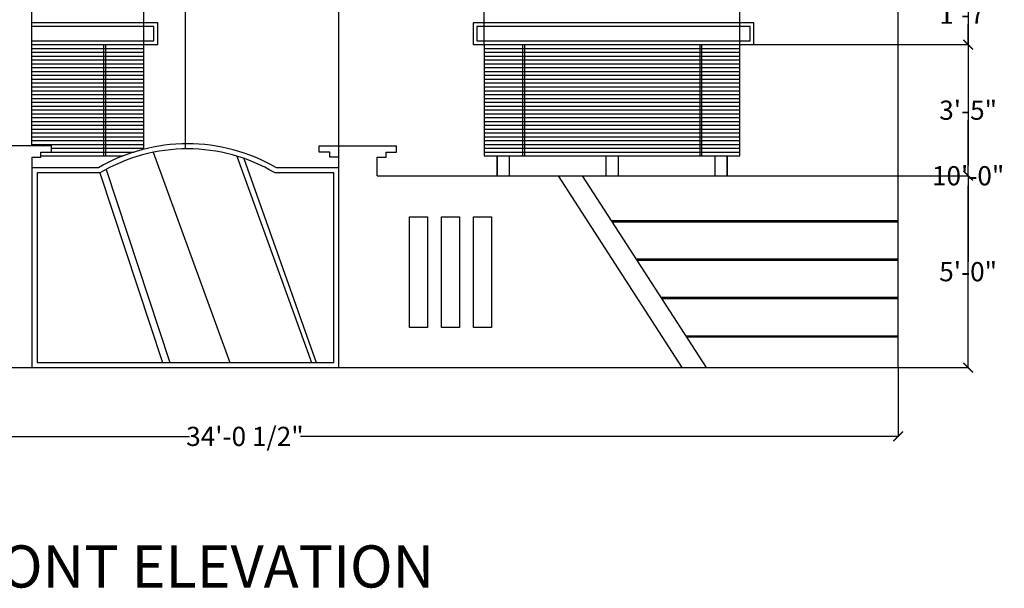
# Model space of a CAD drawing. Units: inches. Extents: x 2278 to 7495, y -71 to 1198.
# Tile 9 of 44: x 4871 to 5179, y -71 to 107. Entities that reach past the tile are written whole.
import ezdxf

# ---------------------------------------------------------------- set-up
doc = ezdxf.new("R2010")
doc.units = ezdxf.units.IN
doc.header["$MEASUREMENT"] = 0
for name, color, linetype, lineweight in [('A-ANNO-DIMS', 2, 'Continuous', 18), ('A-ANNO-TEXT', 7, 'Continuous', 25), ('A-ELEV', 7, 'Continuous', 25)]:
    doc.layers.add(name, color=color, linetype=linetype, lineweight=lineweight)
doc.styles.get("Standard").update_dxf_attribs({"font": 'arial.ttf'})
doc.dimstyles.get("Standard").update_dxf_attribs({"dimtxt": 6, "dimasz": 3, "dimexe": 0.18, "dimexo": 0.0625, "dimgap": 0.09, "dimtad": 0, "dimtih": 1, "dimtoh": 1, "dimdec": 0, "dimzin": 0, "dimdsep": 46, "dimlunit": 3, "dimtxsty": 'Standard', "dimblk": 'ARCHTICK', "dimcen": 0.09, "dimadec": 0, "dimazin": 0, "dimtfac": 1, "dimtdec": 0, "dimtofl": 0, "dimtmove": 0, "dimatfit": 3, "dimfxl": 1, "dimtolj": 1, "dimtzin": 0, "dimarcsym": 0})

# ---------------------------------------------------------------- blocks, each defined once
blk = doc.blocks.new('_ArchTick')
at = {"color": 0, "linetype": 'ByBlock', "const_width": 0.15}
blk.add_lwpolyline([(-0.5, -0.5), (0.5, 0.5)], dxfattribs=at)
blk = doc.blocks.new('*D123')
at = {"layer": 'A-ANNO-DIMS', "color": 0, "lineweight": -2, "transparency": 16777216}
for p, q in [((4736.95, 340.16), (4736.95, -23.43)), ((5145.68, -1.81), (5145.68, -23.43)), ((4736.95, -23.25), (4923.93, -23.25)), ((5145.68, -23.25), (4958.7, -23.25))]:
    blk.add_line(p, q, dxfattribs=at)
at = {"layer": 'Defpoints', "color": 0, "transparency": 16777216}
for p in [(4736.95, 340.22), (5145.68, -1.75), (5145.68, -23.25)]:
    blk.add_point(p, dxfattribs=at)
at = {"layer": 'A-ANNO-DIMS', "color": 0, "lineweight": -2, "transparency": 16777216, "xscale": 3, "yscale": 3, "zscale": 3, "rotation": 180}
blk.add_blockref('_ArchTick', (4736.95, -23.25), dxfattribs=at)
at = {"layer": 'A-ANNO-DIMS', "color": 0, "lineweight": -2, "transparency": 16777216, "xscale": 3, "yscale": 3, "zscale": 3}
blk.add_blockref('_ArchTick', (5145.68, -23.25), dxfattribs=at)
at = {"layer": 'A-ANNO-DIMS', "color": 0, "transparency": 16777216, "insert": (4941.31, -23.25), "char_height": 6, "attachment_point": 5}
blk.add_mtext('\\A1;34\'-0 1/2"', dxfattribs=at)
blk = doc.blocks.new('*D126')
at = {"layer": 'A-ANNO-DIMS', "color": 0, "lineweight": -2, "transparency": 16777216}
for p, q in [((4837.74, 313.27), (4837.74, 361.9)), ((4837.74, 361.72), (4848.14, 361.72)), ((4874.68, 361.72), (4864.27, 361.72)), ((4874.68, 99.32), (4874.68, 361.9))]:
    blk.add_line(p, q, dxfattribs=at)
at = {"layer": 'Defpoints', "color": 0, "transparency": 16777216}
for p in [(4874.68, 361.72), (4837.74, 313.21), (4874.68, 99.25)]:
    blk.add_point(p, dxfattribs=at)
at = {"layer": 'A-ANNO-DIMS', "color": 0, "lineweight": -2, "transparency": 16777216, "xscale": 3, "yscale": 3, "zscale": 3, "rotation": 180}
blk.add_blockref('_ArchTick', (4837.74, 361.72), dxfattribs=at)
at = {"layer": 'A-ANNO-DIMS', "color": 0, "lineweight": -2, "transparency": 16777216, "xscale": 3, "yscale": 3, "zscale": 3}
blk.add_blockref('_ArchTick', (4874.68, 361.72), dxfattribs=at)
at = {"layer": 'A-ANNO-DIMS', "color": 0, "transparency": 16777216, "insert": (4856.21, 361.72), "char_height": 6, "attachment_point": 5}
blk.add_mtext('\\A1;3\'-1"', dxfattribs=at)
blk = doc.blocks.new('*D127')
at = {"layer": 'A-ANNO-DIMS', "color": 0, "lineweight": -2, "transparency": 16777216}
for p, q in [((4874.68, 99.32), (4874.68, 361.9)), ((4874.68, 361.72), (4881.73, 361.72)), ((4909.68, 361.72), (4902.62, 361.72)), ((4909.68, 99.32), (4909.68, 361.9))]:
    blk.add_line(p, q, dxfattribs=at)
at = {"layer": 'Defpoints', "color": 0, "transparency": 16777216}
for p in [(4909.68, 361.72), (4874.68, 99.25), (4909.68, 99.25)]:
    blk.add_point(p, dxfattribs=at)
at = {"layer": 'A-ANNO-DIMS', "color": 0, "lineweight": -2, "transparency": 16777216, "xscale": 3, "yscale": 3, "zscale": 3, "rotation": 180}
blk.add_blockref('_ArchTick', (4874.68, 361.72), dxfattribs=at)
at = {"layer": 'A-ANNO-DIMS', "color": 0, "lineweight": -2, "transparency": 16777216, "xscale": 3, "yscale": 3, "zscale": 3}
blk.add_blockref('_ArchTick', (4909.68, 361.72), dxfattribs=at)
at = {"layer": 'A-ANNO-DIMS', "color": 0, "transparency": 16777216, "insert": (4892.18, 361.72), "char_height": 6, "attachment_point": 5}
blk.add_mtext('\\A1;2\'-11"', dxfattribs=at)
blk = doc.blocks.new('*D128')
at = {"layer": 'A-ANNO-DIMS', "color": 0, "lineweight": -2, "transparency": 16777216}
for p, q in [((4909.68, 99.32), (4909.68, 361.9)), ((4909.68, 361.72), (4932.11, 361.72)), ((4970.68, 361.72), (4948.24, 361.72)), ((4970.68, 60.78), (4970.68, 361.9))]:
    blk.add_line(p, q, dxfattribs=at)
at = {"layer": 'Defpoints', "color": 0, "transparency": 16777216}
for p in [(4970.68, 361.72), (4909.68, 99.25), (4970.68, 60.72)]:
    blk.add_point(p, dxfattribs=at)
at = {"layer": 'A-ANNO-DIMS', "color": 0, "lineweight": -2, "transparency": 16777216, "xscale": 3, "yscale": 3, "zscale": 3, "rotation": 180}
blk.add_blockref('_ArchTick', (4909.68, 361.72), dxfattribs=at)
at = {"layer": 'A-ANNO-DIMS', "color": 0, "lineweight": -2, "transparency": 16777216, "xscale": 3, "yscale": 3, "zscale": 3}
blk.add_blockref('_ArchTick', (4970.68, 361.72), dxfattribs=at)
at = {"layer": 'A-ANNO-DIMS', "color": 0, "transparency": 16777216, "insert": (4940.18, 361.72), "char_height": 6, "attachment_point": 5}
blk.add_mtext('\\A1;5\'-1"', dxfattribs=at)
blk = doc.blocks.new('*D129')
at = {"layer": 'A-ANNO-DIMS', "color": 0, "lineweight": -2, "transparency": 16777216}
for p, q in [((4970.68, 60.78), (4970.68, 361.9)), ((4970.68, 361.72), (4978.37, 361.72)), ((5016.18, 361.72), (5008.48, 361.72)), ((5016.18, 99.32), (5016.18, 361.9))]:
    blk.add_line(p, q, dxfattribs=at)
at = {"layer": 'Defpoints', "color": 0, "transparency": 16777216}
for p in [(5016.18, 361.72), (5016.18, 99.25), (4970.68, 60.72)]:
    blk.add_point(p, dxfattribs=at)
at = {"layer": 'A-ANNO-DIMS', "color": 0, "lineweight": -2, "transparency": 16777216, "xscale": 3, "yscale": 3, "zscale": 3, "rotation": 180}
blk.add_blockref('_ArchTick', (4970.68, 361.72), dxfattribs=at)
at = {"layer": 'A-ANNO-DIMS', "color": 0, "lineweight": -2, "transparency": 16777216, "xscale": 3, "yscale": 3, "zscale": 3}
blk.add_blockref('_ArchTick', (5016.18, 361.72), dxfattribs=at)
at = {"layer": 'A-ANNO-DIMS', "color": 0, "transparency": 16777216, "insert": (4993.43, 361.72), "char_height": 6, "attachment_point": 5}
blk.add_mtext('\\A1;3\'-9 1/2"', dxfattribs=at)
blk = doc.blocks.new('*D130')
at = {"layer": 'A-ANNO-DIMS', "color": 0, "lineweight": -2, "transparency": 16777216}
for p, q in [((5016.18, 99.32), (5016.18, 361.9)), ((5016.18, 361.72), (5048.1, 361.72)), ((5096.18, 361.72), (5064.26, 361.72)), ((5096.18, 99.32), (5096.18, 361.9))]:
    blk.add_line(p, q, dxfattribs=at)
at = {"layer": 'Defpoints', "color": 0, "transparency": 16777216}
for p in [(5096.18, 361.72), (5016.18, 99.25), (5096.18, 99.25)]:
    blk.add_point(p, dxfattribs=at)
at = {"layer": 'A-ANNO-DIMS', "color": 0, "lineweight": -2, "transparency": 16777216, "xscale": 3, "yscale": 3, "zscale": 3, "rotation": 180}
blk.add_blockref('_ArchTick', (5016.18, 361.72), dxfattribs=at)
at = {"layer": 'A-ANNO-DIMS', "color": 0, "lineweight": -2, "transparency": 16777216, "xscale": 3, "yscale": 3, "zscale": 3}
blk.add_blockref('_ArchTick', (5096.18, 361.72), dxfattribs=at)
at = {"layer": 'A-ANNO-DIMS', "color": 0, "transparency": 16777216, "insert": (5056.18, 361.72), "char_height": 6, "attachment_point": 5}
blk.add_mtext('\\A1;6\'-8"', dxfattribs=at)
blk = doc.blocks.new('*D131')
at = {"layer": 'A-ANNO-DIMS', "color": 0, "lineweight": -2, "transparency": 16777216}
for p, q in [((5096.18, 99.32), (5096.18, 361.9)), ((5096.18, 361.72), (5105.75, 361.72)), ((5145.68, 361.72), (5136.1, 361.72)), ((5145.68, 118.32), (5145.68, 361.9))]:
    blk.add_line(p, q, dxfattribs=at)
at = {"layer": 'Defpoints', "color": 0, "transparency": 16777216}
for p in [(5145.68, 361.72), (5145.68, 118.25), (5096.18, 99.25)]:
    blk.add_point(p, dxfattribs=at)
at = {"layer": 'A-ANNO-DIMS', "color": 0, "lineweight": -2, "transparency": 16777216, "xscale": 3, "yscale": 3, "zscale": 3, "rotation": 180}
blk.add_blockref('_ArchTick', (5096.18, 361.72), dxfattribs=at)
at = {"layer": 'A-ANNO-DIMS', "color": 0, "lineweight": -2, "transparency": 16777216, "xscale": 3, "yscale": 3, "zscale": 3}
blk.add_blockref('_ArchTick', (5145.68, 361.72), dxfattribs=at)
at = {"layer": 'A-ANNO-DIMS', "color": 0, "transparency": 16777216, "insert": (5120.93, 361.72), "char_height": 6, "attachment_point": 5}
blk.add_mtext('\\A1;4\'-1 1/2"', dxfattribs=at)
blk = doc.blocks.new('*D136')
at = {"layer": 'A-ANNO-DIMS', "color": 0, "lineweight": -2, "transparency": 16777216}
for p, q in [((5145.74, 58.25), (5167.75, 58.25)), ((5167.57, 58.25), (5167.57, 31.41)), ((5167.57, -1.75), (5167.57, 25.1)), ((5145.74, -1.75), (5167.75, -1.75))]:
    blk.add_line(p, q, dxfattribs=at)
at = {"layer": 'Defpoints', "color": 0, "transparency": 16777216}
for p in [(5145.68, 58.25), (5167.57, 58.25), (5145.68, -1.75)]:
    blk.add_point(p, dxfattribs=at)
at = {"layer": 'A-ANNO-DIMS', "color": 0, "lineweight": -2, "transparency": 16777216, "xscale": 3, "yscale": 3, "zscale": 3}
for p, rotation in [((5167.57, 58.25), 90), ((5167.57, -1.75), 270)]:
    blk.add_blockref('_ArchTick', p, dxfattribs=dict(at, rotation=rotation))
at = {"layer": 'A-ANNO-DIMS', "color": 0, "transparency": 16777216, "insert": (5167.57, 28.25), "char_height": 6, "attachment_point": 5}
blk.add_mtext('\\A1;5\'-0"', dxfattribs=at)
blk = doc.blocks.new('*D137')
at = {"layer": 'A-ANNO-DIMS', "color": 0, "lineweight": -2, "transparency": 16777216}
for p, q in [((5096.24, 99.25), (5167.75, 99.25)), ((5167.57, 99.25), (5167.57, 81.91)), ((5167.57, 58.25), (5167.57, 75.6)), ((5145.74, 58.25), (5167.75, 58.25))]:
    blk.add_line(p, q, dxfattribs=at)
at = {"layer": 'Defpoints', "color": 0, "transparency": 16777216}
for p in [(5096.18, 99.25), (5167.57, 99.25), (5145.68, 58.25)]:
    blk.add_point(p, dxfattribs=at)
at = {"layer": 'A-ANNO-DIMS', "color": 0, "lineweight": -2, "transparency": 16777216, "xscale": 3, "yscale": 3, "zscale": 3}
for p, rotation in [((5167.57, 99.25), 90), ((5167.57, 58.25), 270)]:
    blk.add_blockref('_ArchTick', p, dxfattribs=dict(at, rotation=rotation))
at = {"layer": 'A-ANNO-DIMS', "color": 0, "transparency": 16777216, "insert": (5167.57, 78.75), "char_height": 6, "attachment_point": 5}
blk.add_mtext('\\A1;3\'-5"', dxfattribs=at)
blk = doc.blocks.new('*D138')
at = {"layer": 'A-ANNO-DIMS', "color": 0, "lineweight": -2, "transparency": 16777216}
for p, q in [((5145.74, 118.25), (5167.75, 118.25)), ((5167.57, 118.25), (5167.57, 111.86)), ((5167.57, 99.25), (5167.57, 105.65)), ((5096.24, 99.25), (5167.75, 99.25))]:
    blk.add_line(p, q, dxfattribs=at)
at = {"layer": 'Defpoints', "color": 0, "transparency": 16777216}
for p in [(5145.68, 118.25), (5167.57, 118.25), (5096.18, 99.25)]:
    blk.add_point(p, dxfattribs=at)
at = {"layer": 'A-ANNO-DIMS', "color": 0, "lineweight": -2, "transparency": 16777216, "xscale": 3, "yscale": 3, "zscale": 3}
for p, rotation in [((5167.57, 118.25), 90), ((5167.57, 99.25), 270)]:
    blk.add_blockref('_ArchTick', p, dxfattribs=dict(at, rotation=rotation))
at = {"layer": 'A-ANNO-DIMS', "color": 0, "transparency": 16777216, "insert": (5167.57, 108.75), "char_height": 6, "attachment_point": 5}
blk.add_mtext('\\A1;1\'-7"', dxfattribs=at)
blk = doc.blocks.new('*D143')
at = {"layer": 'A-ANNO-DIMS', "color": 0, "lineweight": -2, "transparency": 16777216}
for p, q in [((5145.74, 118.25), (5167.75, 118.25)), ((5167.57, 118.25), (5167.57, 61.41)), ((5167.57, -1.75), (5167.57, 55.1)), ((5145.74, -1.75), (5167.75, -1.75))]:
    blk.add_line(p, q, dxfattribs=at)
at = {"layer": 'Defpoints', "color": 0, "transparency": 16777216}
for p in [(5145.68, 118.25), (5167.57, 118.25), (5145.68, -1.75)]:
    blk.add_point(p, dxfattribs=at)
at = {"layer": 'A-ANNO-DIMS', "color": 0, "lineweight": -2, "transparency": 16777216, "xscale": 3, "yscale": 3, "zscale": 3}
for p, rotation in [((5167.57, 118.25), 90), ((5167.57, -1.75), 270)]:
    blk.add_blockref('_ArchTick', p, dxfattribs=dict(at, rotation=rotation))
at = {"layer": 'A-ANNO-DIMS', "color": 0, "transparency": 16777216, "insert": (5167.57, 58.25), "char_height": 6, "attachment_point": 5}
blk.add_mtext('\\A1;10\'-0"', dxfattribs=at)

msp = doc.modelspace()

# ---------------------------------------------------------------- linework, layer by layer
at = {"layer": 'A-ELEV'}
for p, q in [((4922.68, 66.66), (4922.68, 244.25)), ((5145.68, -1.75), (5145.68, 161.58)), ((4970.68, 67.61), (4970.68, 124.25)), ((4874.68, 67.61), (4874.68, 118.25)), ((4874.68, 99.25), (4909.68, 99.25)), ((4897.08, 99.25), (4897.08, 64.45)), ((4897.08, 99.25), (4897.08, 65.65)), ((4897.08, 99.25), (4897.08, 65.65)), ((4897.08, 99.25), (4897.08, 65.65)), ((4897.68, 99.25), (4897.68, 64.45)), ((4897.68, 99.25), (4897.68, 65.65)), ((4897.68, 99.25), (4897.68, 65.65)), ((4897.68, 99.25), (4897.68, 65.65)), ((4909.68, 66.54), (4909.68, 99.25)), ((5016.18, 99.25), (5096.18, 99.25)), ((5016.18, 99.25), (5016.18, 64.45)), ((5028.18, 99.25), (5028.18, 64.45)), ((5028.18, 99.25), (5028.18, 65.65)), ((5028.18, 99.25), (5028.18, 65.65)), ((5028.18, 99.25), (5028.18, 65.65)), ((5028.78, 99.25), (5028.78, 64.45)), ((5028.78, 99.25), (5028.78, 65.65)), ((5028.78, 99.25), (5028.78, 65.65)), ((5028.78, 99.25), (5028.78, 65.65)), ((5083.58, 99.25), (5083.58, 64.45)), ((5083.58, 99.25), (5083.58, 65.65)), ((5083.58, 99.25), (5083.58, 65.65)), ((5083.58, 99.25), (5083.58, 65.65)), ((5084.18, 99.25), (5084.18, 64.45)), ((5084.18, 99.25), (5084.18, 65.65)), ((5084.18, 99.25), (5084.18, 65.65)), ((5084.18, 99.25), (5084.18, 65.65)), ((5096.18, 64.45), (5096.18, 99.25)), ((4874.68, 98.05), (4909.68, 98.05)), ((4874.68, 96.85), (4909.68, 96.85)), ((4874.68, 95.65), (4909.68, 95.65)), ((5016.18, 98.05), (5096.18, 98.05)), ((5016.18, 96.85), (5096.18, 96.85)), ((5016.18, 95.65), (5096.18, 95.65)), ((4874.68, 94.45), (4909.68, 94.45)), ((4874.68, 93.25), (4909.68, 93.25)), ((5016.18, 94.45), (5096.18, 94.45)), ((5016.18, 93.25), (5096.18, 93.25)), ((4874.68, 92.05), (4909.68, 92.05)), ((4874.68, 90.85), (4909.68, 90.85)), ((4874.68, 89.65), (4909.68, 89.65)), ((5016.18, 92.05), (5096.18, 92.05)), ((5016.18, 90.85), (5096.18, 90.85)), ((5016.18, 89.65), (5096.18, 89.65)), ((4874.68, 88.45), (4909.68, 88.45)), ((4874.68, 87.25), (4909.68, 87.25)), ((5016.18, 88.45), (5096.18, 88.45)), ((5016.18, 87.25), (5096.18, 87.25)), ((4874.68, 86.05), (4909.68, 86.05)), ((4874.68, 84.85), (4909.68, 84.85)), ((4874.68, 83.65), (4909.68, 83.65)), ((5016.18, 86.05), (5096.18, 86.05)), ((5016.18, 84.85), (5096.18, 84.85)), ((5016.18, 83.65), (5096.18, 83.65)), ((4874.68, 82.45), (4909.68, 82.45)), ((4874.68, 81.25), (4909.68, 81.25)), ((5016.18, 82.45), (5096.18, 82.45)), ((5016.18, 81.25), (5096.18, 81.25)), ((4874.68, 80.05), (4909.68, 80.05)), ((4874.68, 78.85), (4909.68, 78.85)), ((4874.68, 77.65), (4909.68, 77.65)), ((5016.18, 80.05), (5096.18, 80.05)), ((5016.18, 78.85), (5096.18, 78.85)), ((5016.18, 77.65), (5096.18, 77.65)), ((4874.68, 76.45), (4909.68, 76.45)), ((4874.68, 75.25), (4909.68, 75.25)), ((4874.68, 74.05), (4909.68, 74.05)), ((5016.18, 76.45), (5096.18, 76.45)), ((5016.18, 75.25), (5096.18, 75.25)), ((5016.18, 74.05), (5096.18, 74.05)), ((4874.68, 72.85), (4909.68, 72.85)), ((4874.68, 71.65), (4909.68, 71.65)), ((5016.18, 72.85), (5096.18, 72.85)), ((5016.18, 71.65), (5096.18, 71.65)), ((4874.68, 70.45), (4909.68, 70.45)), ((4874.68, 69.25), (4909.68, 69.25)), ((4874.68, 68.05), (4909.68, 68.05)), ((5016.18, 70.45), (5096.18, 70.45)), ((5016.18, 69.25), (5096.18, 69.25)), ((5016.18, 68.05), (5096.18, 68.05)), ((4880.77, 67.61), (4856.59, 67.61)), ((4877.51, 64.1), (4877.51, 65.61)), ((4877.51, 65.61), (4880.77, 65.61)), ((4880.77, 65.61), (4880.77, 67.61)), ((4880.77, 66.85), (4909.68, 66.85)), ((4880.77, 65.65), (4906.57, 65.65)), ((4912.62, 65.58), (4936.59, -0.15)), ((4964.59, 65.61), (4964.59, 67.61)), ((4964.59, 67.61), (4988.77, 67.61)), ((4967.85, 65.61), (4964.59, 65.61)), ((4967.85, 64.1), (4967.85, 65.61)), ((4985.51, 64.1), (4985.51, 65.61)), ((4985.51, 65.61), (4988.77, 65.61)), ((4988.77, 65.61), (4988.77, 67.61)), ((5016.18, 66.85), (5096.18, 66.85)), ((5016.18, 65.65), (5096.18, 65.65)), ((4874.68, 64.1), (4877.51, 64.1)), ((4874.68, 64.1), (4874.68, 60.72)), ((4877.51, 64.45), (4903.2, 64.45)), ((4938.76, 64.39), (4962.09, -0.15)), ((4940.97, 63.67), (4963.65, -0.15)), ((4970.68, 64.1), (4967.85, 64.1)), ((4970.68, 60.72), (4970.68, 64.1)), ((4982.68, 58.25), (4982.68, 64.1)), ((4982.68, 64.1), (4985.51, 64.1)), ((5016.18, 64.45), (5096.18, 64.45)), ((5020.18, 64.45), (5020.18, 58.25)), ((5020.18, 64.45), (5020.18, 58.25)), ((5020.18, 64.45), (5020.18, 58.25)), ((5020.18, 58.25), (5020.18, 64.45)), ((5020.18, 58.25), (5020.18, 64.45)), ((5023.97, 64.45), (5023.97, 58.25)), ((5023.97, 64.45), (5023.97, 58.25)), ((5054.28, 58.25), (5054.28, 64.45)), ((5054.28, 58.25), (5054.28, 64.45)), ((5058.07, 64.45), (5058.07, 58.25)), ((5058.07, 64.45), (5058.07, 58.25)), ((5088.39, 58.25), (5088.39, 64.45)), ((5088.39, 58.25), (5088.39, 64.45)), ((5092.18, 64.45), (5092.18, 58.25)), ((5092.18, 64.45), (5092.18, 58.25)), ((5092.18, 64.45), (5092.18, 58.25)), ((5092.18, 64.45), (5092.18, 58.25)), ((5092.18, 64.45), (5092.18, 58.25)), ((5092.18, 58.25), (5092.18, 64.45)), ((4874.68, 60.72), (4874.68, -1.75)), ((4895.93, 59.12), (4915.52, -0.15)), ((4897.92, 60.25), (4917.86, -0.15)), ((4982.68, 58.25), (5145.68, 58.25)), ((5039.26, 58.25), (5078, -1.75)), ((5046.83, 58.25), (5085.57, -1.75)), ((5056.01, 44.24), (5145.68, 44.24)), ((5056.01, 44.24), (5056.01, 44.04)), ((5056.14, 43.84), (5145.68, 43.84)), ((5145.68, 43.84), (5145.68, 44.24)), ((5063.63, 32.24), (5145.68, 32.24)), ((5063.89, 31.84), (5145.68, 31.84)), ((5071.38, 20.24), (5145.68, 20.24)), ((5071.63, 19.84), (5145.68, 19.84)), ((5079.12, 8.24), (5145.68, 8.24)), ((5079.38, 7.84), (5145.68, 7.84)), ((4742.68, -1.75), (5145.68, -1.75))]:
    msp.add_line(p, q, dxfattribs=at)
for points in [[(4874.68, 99.25), (4914.03, 99.25), (4914.03, 106.1), (4874.68, 106.1)], [(4874.68, 100.45), (4912.83, 100.45), (4912.83, 104.9), (4874.68, 104.9)], [(4895.49, 60.72), (4874.68, 60.72), (4874.68, -1.75), (4970.68, -1.75), (4970.68, 60.72), (4951.16, 60.72)], [(4895.93, 59.12), (4876.28, 59.12), (4876.28, -0.15), (4969.08, -0.15), (4969.08, 59.12), (4950.73, 59.12)]]:
    msp.add_lwpolyline(points, dxfattribs=at)
for points in [[(5012.69, 99.25), (5100.53, 99.25), (5100.53, 106.1), (5012.69, 106.1)], [(5013.89, 100.45), (5099.33, 100.45), (5099.33, 104.9), (5013.89, 104.9)], [(4992.85, 45.42), (4998.43, 45.42), (4998.43, 10.78), (4992.85, 10.78)], [(5002.85, 45.42), (5008.43, 45.42), (5008.43, 10.78), (5002.85, 10.78)], [(5012.85, 45.42), (5018.43, 45.42), (5018.43, 10.78), (5012.85, 10.78)]]:
    msp.add_lwpolyline(points, close=True, dxfattribs=at)
for radius, start, end in [(55.14, 59.6802, 120.3198), (53.54, 59.2195, 120.7805)]:
    msp.add_arc((4923.33, 13.12), radius, start, end, dxfattribs=at)

# ---------------------------------------------------------------- texts
at = {"layer": 'A-ANNO-TEXT'}
msp.add_text('FRONT ELEVATION', height=13.1927, dxfattribs=at).set_placement((4843.31, -70.51))

# ---------------------------------------------------------------- dimensions: what is measured, and where the dimension line sits
at = {"layer": 'A-ANNO-DIMS'}
for base, p1, p2, picture, middle in [((5016.18, 361.72), (4970.68, 60.72), (5016.18, 99.25), '*D129', (4993.43, 361.72)), ((5145.68, 361.72), (5096.18, 99.25), (5145.68, 118.25), '*D131', (5120.93, 361.72)), ((4874.68, 361.72), (4837.74, 313.21), (4874.68, 99.25), '*D126', (4856.21, 361.72)), ((4909.68, 361.72), (4874.68, 99.25), (4909.68, 99.25), '*D127', (4892.18, 361.72)), ((4970.68, 361.72), (4909.68, 99.25), (4970.68, 60.72), '*D128', (4940.18, 361.72)), ((5096.18, 361.72), (5016.18, 99.25), (5096.18, 99.25), '*D130', (5056.18, 361.72)), ((5145.68, -23.25), (4736.95, 340.22), (5145.68, -1.75), '*D123', (4941.31, -23.25))]:
    dim = msp.add_linear_dim(base=base, p1=p1, p2=p2, dimstyle='Standard', override={"dimdec": 1, "dimlfac": 1, "dimrnd": 0, "dimzin": 1, "dimdsep": 46, "dimlunit": 4, "dimfrac": 2}, dxfattribs=at)
    dim.commit()
    dim.dimension.update_dxf_attribs({"geometry": picture, "text_midpoint": middle})
for base, p1, p2, picture, middle in [((5167.57, 118.25), (5096.18, 99.25), (5145.68, 118.25), '*D138', (5167.57, 108.75)), ((5167.57, 118.25), (5145.68, -1.75), (5145.68, 118.25), '*D143', (5167.57, 58.25)), ((5167.57, 99.25), (5145.68, 58.25), (5096.18, 99.25), '*D137', (5167.57, 78.75)), ((5167.57, 58.25), (5145.68, -1.75), (5145.68, 58.25), '*D136', (5167.57, 28.25))]:
    dim = msp.add_linear_dim(base=base, p1=p1, p2=p2, angle=90, dimstyle='Standard', override={"dimdec": 1, "dimlfac": 1, "dimrnd": 0, "dimzin": 1, "dimdsep": 46, "dimlunit": 4, "dimfrac": 2}, dxfattribs=at)
    dim.commit()
    dim.dimension.update_dxf_attribs({"geometry": picture, "text_midpoint": middle})

doc.saveas('drawing.dxf')
